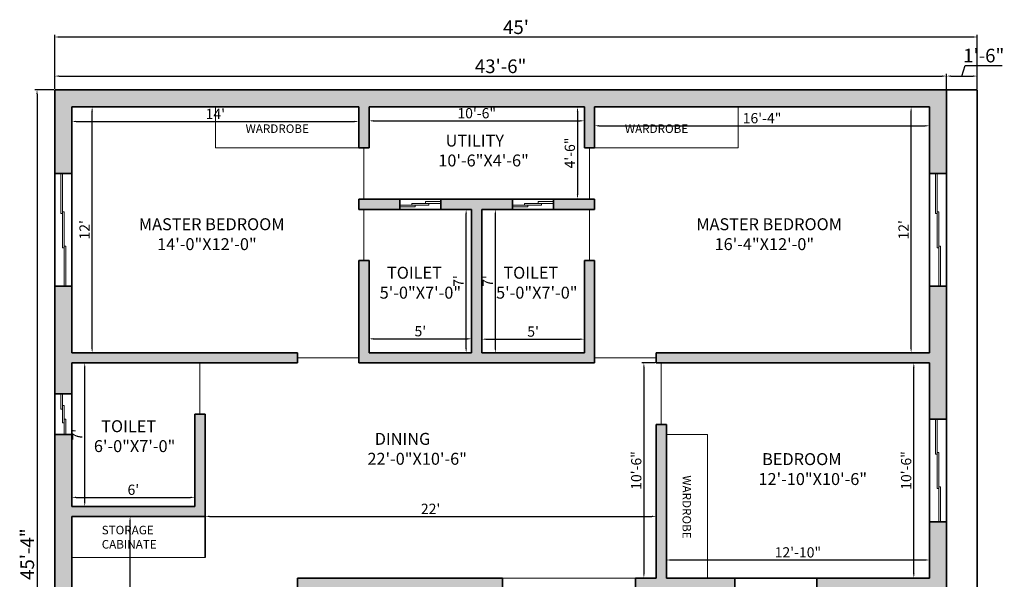
# Model space of a CAD drawing. Units: inches. Extents: x 3491 to 6898, y 1360 to 2019.
# Tile 7 of 9: x 5693 to 6269, y 1686 to 2013. Entities that reach past the tile are written whole.
import ezdxf

# ---------------------------------------------------------------- set-up
doc = ezdxf.new("R2010")
doc.units = ezdxf.units.IN
for name, color, linetype, lineweight in [('A-ANNO-DIMS', 2, 'Continuous', 18), ('A-ANNO-TEXT', 7, 'Continuous', 18), ('A-AREA-IDEN', 7, 'Continuous', 18), ('A-DOOR', 4, 'Continuous', 18), ('A-FLOR-CASE', 8, 'Continuous', 18), ('A-GLAZ', 5, 'Continuous', 18), ('A-WALL', 7, 'Continuous', 35), ('A-WALL-PATT', 8, 'Continuous', 13)]:
    doc.layers.add(name, color=color, linetype=linetype, lineweight=lineweight)
doc.layers.add('A-WALL-OPEN', color=251, linetype='Continuous', lineweight=13, true_color=0x636466)
doc.styles.get("Standard").update_dxf_attribs({"font": 'arial.ttf'})
doc.dimstyles.new('ISO-25', dxfattribs={"dimtxt": 8, "dimasz": 2.5, "dimexe": 1.25, "dimexo": 0.625, "dimtad": 1, "dimdec": 1, "dimlunit": 3, "dimtxsty": 'Standard', "dimcen": 2.5, "dimclrt": 1, "dimadec": 0, "dimazin": 0, "dimtfac": 1, "dimtdec": 1, "dimtmove": 0, "dimatfit": 3, "dimfxl": 1, "dimarcsym": 0})

# ---------------------------------------------------------------- blocks, each defined once
blk = doc.blocks.new('*D51')
at = {"layer": 'A-ANNO-DIMS', "color": 0, "lineweight": -2, "transparency": 16777216}
for p, q in [((5713.61, 1972.99), (5713.61, 1981.69)), ((5716.11, 1980.44), (6233.11, 1980.44)), ((6235.61, 1972.99), (6235.61, 1981.69))]:
    blk.add_line(p, q, dxfattribs=at)
at = {"layer": 'A-ANNO-DIMS', "color": 0, "transparency": 16777216}
for points in [[(5716.11, 1980.85), (5716.11, 1980.02), (5713.61, 1980.44)], [(6233.11, 1980.85), (6233.11, 1980.02), (6235.61, 1980.44)]]:
    blk.add_solid(points, dxfattribs=at)
at = {"layer": 'Defpoints', "color": 0, "transparency": 16777216}
for p in [(6235.61, 1980.44), (5713.61, 1972.37), (6235.61, 1972.37)]:
    blk.add_point(p, dxfattribs=at)
at = {"layer": 'A-ANNO-DIMS', "color": 0, "transparency": 16777216, "insert": (5974.61, 1985.15), "char_height": 8, "attachment_point": 5}
blk.add_mtext('43\'-6"', dxfattribs=at)
blk = doc.blocks.new('*D52')
at = {"layer": 'A-ANNO-DIMS', "color": 0, "lineweight": -2, "transparency": 16777216}
for p, q in [((6244.61, 1980.44), (6246.49, 1986.71)), ((6246.49, 1986.71), (6268.26, 1986.71)), ((6235.61, 1972.99), (6235.61, 1981.69)), ((6238.11, 1980.44), (6251.11, 1980.44)), ((6253.61, 1972.99), (6253.61, 1981.69))]:
    blk.add_line(p, q, dxfattribs=at)
at = {"layer": 'A-ANNO-DIMS', "color": 0, "transparency": 16777216}
for points in [[(6238.11, 1980.85), (6238.11, 1980.02), (6235.61, 1980.44)], [(6251.11, 1980.85), (6251.11, 1980.02), (6253.61, 1980.44)]]:
    blk.add_solid(points, dxfattribs=at)
at = {"layer": 'Defpoints', "color": 0, "transparency": 16777216}
for p in [(6253.61, 1980.44), (6235.61, 1972.37), (6253.61, 1972.37)]:
    blk.add_point(p, dxfattribs=at)
at = {"layer": 'A-ANNO-DIMS', "color": 0, "transparency": 16777216, "insert": (6257.38, 1991.42), "char_height": 8, "attachment_point": 5}
blk.add_mtext('1\'-6"', dxfattribs=at)
blk = doc.blocks.new('*D32')
at = {"layer": 'A-ANNO-DIMS', "color": 0, "lineweight": -2, "transparency": 16777216}
for p, q in [((5713.61, 1972.99), (5713.61, 2004.59)), ((5716.11, 2003.34), (6251.11, 2003.34)), ((6253.61, 1972.99), (6253.61, 2004.59))]:
    blk.add_line(p, q, dxfattribs=at)
at = {"layer": 'A-ANNO-DIMS', "color": 0, "transparency": 16777216}
for points in [[(5716.11, 2003.76), (5716.11, 2002.92), (5713.61, 2003.34)], [(6251.11, 2003.76), (6251.11, 2002.92), (6253.61, 2003.34)]]:
    blk.add_solid(points, dxfattribs=at)
at = {"layer": 'Defpoints', "color": 0, "transparency": 16777216}
for p in [(6253.61, 2003.34), (5713.61, 1972.37), (6253.61, 1972.37)]:
    blk.add_point(p, dxfattribs=at)
at = {"layer": 'A-ANNO-DIMS', "color": 0, "transparency": 16777216, "insert": (5983.61, 2008.03), "char_height": 8, "attachment_point": 5}
blk.add_mtext("45'", dxfattribs=at)
blk = doc.blocks.new('*D53')
at = {"layer": 'A-ANNO-DIMS', "color": 0, "lineweight": -2, "transparency": 16777216}
for p, q in [((5712.99, 1972.37), (5701.98, 1972.37)), ((5703.23, 1969.87), (5703.23, 1430.87)), ((5712.99, 1428.37), (5701.98, 1428.37))]:
    blk.add_line(p, q, dxfattribs=at)
at = {"layer": 'A-ANNO-DIMS', "color": 0, "transparency": 16777216}
for points in [[(5702.81, 1969.87), (5703.65, 1969.87), (5703.23, 1972.37)], [(5702.81, 1430.87), (5703.65, 1430.87), (5703.23, 1428.37)]]:
    blk.add_solid(points, dxfattribs=at)
at = {"layer": 'Defpoints', "color": 0, "transparency": 16777216}
for p in [(5713.61, 1972.37), (5703.23, 1428.37), (5713.61, 1428.37)]:
    blk.add_point(p, dxfattribs=at)
at = {"layer": 'A-ANNO-DIMS', "color": 0, "transparency": 16777216, "insert": (5698.54, 1700.37), "char_height": 8, "attachment_point": 5, "rotation": 90}
blk.add_mtext('45\'-4"', dxfattribs=at)
blk = doc.blocks.new('*D54')
at = {"layer": 'A-ANNO-DIMS', "color": 0, "lineweight": -2, "transparency": 16777216}
for p, q in [((5723.61, 1728.99), (5723.61, 1734.88)), ((5795.61, 1728.99), (5795.61, 1734.88)), ((5726.11, 1733.63), (5793.11, 1733.63))]:
    blk.add_line(p, q, dxfattribs=at)
at = {"layer": 'A-ANNO-DIMS', "color": 0, "transparency": 16777216}
for points in [[(5726.11, 1734.05), (5726.11, 1733.21), (5723.61, 1733.63)], [(5793.11, 1734.05), (5793.11, 1733.21), (5795.61, 1733.63)]]:
    blk.add_solid(points, dxfattribs=at)
at = {"layer": 'Defpoints', "color": 0, "transparency": 16777216}
for p in [(5795.61, 1733.63), (5723.61, 1728.37), (5795.61, 1728.37)]:
    blk.add_point(p, dxfattribs=at)
at = {"layer": 'A-ANNO-DIMS', "color": 0, "transparency": 16777216, "insert": (5759.61, 1737.32), "char_height": 6, "attachment_point": 5}
blk.add_mtext("6'", dxfattribs=at)
blk = doc.blocks.new('*D55')
at = {"layer": 'A-ANNO-DIMS', "color": 0, "lineweight": -2, "transparency": 16777216}
for p, q in [((5724.24, 1812.37), (5732.4, 1812.37)), ((5731.15, 1730.87), (5731.15, 1809.87)), ((5724.24, 1728.37), (5732.4, 1728.37))]:
    blk.add_line(p, q, dxfattribs=at)
at = {"layer": 'A-ANNO-DIMS', "color": 0, "transparency": 16777216}
for points in [[(5730.73, 1809.87), (5731.57, 1809.87), (5731.15, 1812.37)], [(5730.73, 1730.87), (5731.57, 1730.87), (5731.15, 1728.37)]]:
    blk.add_solid(points, dxfattribs=at)
at = {"layer": 'Defpoints', "color": 0, "transparency": 16777216}
for p in [(5723.61, 1812.37), (5731.15, 1812.37), (5723.61, 1728.37)]:
    blk.add_point(p, dxfattribs=at)
at = {"layer": 'A-ANNO-DIMS', "color": 0, "transparency": 16777216, "insert": (5727.53, 1770.37), "char_height": 6, "attachment_point": 5, "rotation": 90}
blk.add_mtext("7'", dxfattribs=at)
blk = doc.blocks.new('*D56')
at = {"layer": 'A-ANNO-DIMS', "color": 0, "lineweight": -2, "transparency": 16777216}
for p, q in [((5724.24, 1962.37), (5736.74, 1962.37)), ((5735.49, 1820.87), (5735.49, 1959.87)), ((5724.24, 1818.37), (5736.74, 1818.37))]:
    blk.add_line(p, q, dxfattribs=at)
at = {"layer": 'A-ANNO-DIMS', "color": 0, "transparency": 16777216}
for points in [[(5735.07, 1959.87), (5735.9, 1959.87), (5735.49, 1962.37)], [(5735.07, 1820.87), (5735.9, 1820.87), (5735.49, 1818.37)]]:
    blk.add_solid(points, dxfattribs=at)
at = {"layer": 'Defpoints', "color": 0, "transparency": 16777216}
for p in [(5723.61, 1962.37), (5735.49, 1962.37), (5723.61, 1818.37)]:
    blk.add_point(p, dxfattribs=at)
at = {"layer": 'A-ANNO-DIMS', "color": 0, "transparency": 16777216, "insert": (5731.85, 1890.37), "char_height": 6, "attachment_point": 5, "rotation": 90}
blk.add_mtext("12'", dxfattribs=at)
blk = doc.blocks.new('*D57')
at = {"layer": 'A-ANNO-DIMS', "color": 0, "lineweight": -2, "transparency": 16777216}
for p, q in [((5723.61, 1961.74), (5723.61, 1952.59)), ((5891.61, 1961.74), (5891.61, 1952.59)), ((5726.11, 1953.84), (5889.11, 1953.84))]:
    blk.add_line(p, q, dxfattribs=at)
at = {"layer": 'A-ANNO-DIMS', "color": 0, "transparency": 16777216}
for points in [[(5726.11, 1954.26), (5726.11, 1953.42), (5723.61, 1953.84)], [(5889.11, 1954.26), (5889.11, 1953.42), (5891.61, 1953.84)]]:
    blk.add_solid(points, dxfattribs=at)
at = {"layer": 'Defpoints', "color": 0, "transparency": 16777216}
for p in [(5723.61, 1962.37), (5891.61, 1962.37), (5891.61, 1953.84)]:
    blk.add_point(p, dxfattribs=at)
at = {"layer": 'A-ANNO-DIMS', "color": 0, "transparency": 16777216, "insert": (5807.61, 1957.48), "char_height": 6, "attachment_point": 5}
blk.add_mtext("14'", dxfattribs=at)
blk = doc.blocks.new('*D58')
at = {"layer": 'A-ANNO-DIMS', "color": 0, "lineweight": -2, "transparency": 16777216}
for p, q in [((5897.61, 1961.74), (5897.61, 1952.97)), ((6023.61, 1961.74), (6023.61, 1952.97)), ((5900.11, 1954.22), (6021.11, 1954.22))]:
    blk.add_line(p, q, dxfattribs=at)
at = {"layer": 'A-ANNO-DIMS', "color": 0, "transparency": 16777216}
for points in [[(5900.11, 1954.64), (5900.11, 1953.81), (5897.61, 1954.22)], [(6021.11, 1954.64), (6021.11, 1953.81), (6023.61, 1954.22)]]:
    blk.add_solid(points, dxfattribs=at)
at = {"layer": 'Defpoints', "color": 0, "transparency": 16777216}
for p in [(5897.61, 1962.37), (6023.61, 1962.37), (6023.61, 1954.22)]:
    blk.add_point(p, dxfattribs=at)
at = {"layer": 'A-ANNO-DIMS', "color": 0, "transparency": 16777216, "insert": (5960.61, 1957.91), "char_height": 6, "attachment_point": 5}
blk.add_mtext('10\'-6"', dxfattribs=at)
blk = doc.blocks.new('*D59')
at = {"layer": 'A-ANNO-DIMS', "color": 0, "lineweight": -2, "transparency": 16777216}
for p, q in [((6029.61, 1961.74), (6029.61, 1950.07)), ((6225.61, 1961.74), (6225.61, 1950.07)), ((6032.11, 1951.32), (6223.11, 1951.32))]:
    blk.add_line(p, q, dxfattribs=at)
at = {"layer": 'A-ANNO-DIMS', "color": 0, "transparency": 16777216}
for points in [[(6032.11, 1951.73), (6032.11, 1950.9), (6029.61, 1951.32)], [(6223.11, 1951.73), (6223.11, 1950.9), (6225.61, 1951.32)]]:
    blk.add_solid(points, dxfattribs=at)
at = {"layer": 'Defpoints', "color": 0, "transparency": 16777216}
for p in [(6029.61, 1962.37), (6225.61, 1962.37), (6225.61, 1951.32)]:
    blk.add_point(p, dxfattribs=at)
at = {"layer": 'A-ANNO-DIMS', "color": 0, "transparency": 16777216, "insert": (6127.61, 1955), "char_height": 6, "attachment_point": 5}
blk.add_mtext('16\'-4"', dxfattribs=at)
blk = doc.blocks.new('*D60')
at = {"layer": 'A-ANNO-DIMS', "color": 0, "lineweight": -2, "transparency": 16777216}
for p, q in [((6224.99, 1962.37), (6213.63, 1962.37)), ((6214.88, 1820.87), (6214.88, 1959.87)), ((6224.99, 1818.37), (6213.63, 1818.37))]:
    blk.add_line(p, q, dxfattribs=at)
at = {"layer": 'A-ANNO-DIMS', "color": 0, "transparency": 16777216}
for points in [[(6214.47, 1959.87), (6215.3, 1959.87), (6214.88, 1962.37)], [(6214.47, 1820.87), (6215.3, 1820.87), (6214.88, 1818.37)]]:
    blk.add_solid(points, dxfattribs=at)
at = {"layer": 'Defpoints', "color": 0, "transparency": 16777216}
for p in [(6214.88, 1962.37), (6225.61, 1962.37), (6225.61, 1818.37)]:
    blk.add_point(p, dxfattribs=at)
at = {"layer": 'A-ANNO-DIMS', "color": 0, "transparency": 16777216, "insert": (6211.25, 1890.37), "char_height": 6, "attachment_point": 5, "rotation": 90}
blk.add_mtext("12'", dxfattribs=at)
blk = doc.blocks.new('*D61')
at = {"layer": 'A-ANNO-DIMS', "color": 0, "lineweight": -2, "transparency": 16777216}
for p, q in [((6071.61, 1686.99), (6071.61, 1698.19)), ((6074.11, 1696.94), (6223.11, 1696.94)), ((6225.61, 1686.99), (6225.61, 1698.19))]:
    blk.add_line(p, q, dxfattribs=at)
at = {"layer": 'A-ANNO-DIMS', "color": 0, "transparency": 16777216}
for points in [[(6074.11, 1697.36), (6074.11, 1696.53), (6071.61, 1696.94)], [(6223.11, 1697.36), (6223.11, 1696.53), (6225.61, 1696.94)]]:
    blk.add_solid(points, dxfattribs=at)
at = {"layer": 'Defpoints', "color": 0, "transparency": 16777216}
for p in [(6225.61, 1696.94), (6071.61, 1686.37), (6225.61, 1686.37)]:
    blk.add_point(p, dxfattribs=at)
at = {"layer": 'A-ANNO-DIMS', "color": 0, "transparency": 16777216, "insert": (6148.61, 1700.63), "char_height": 6, "attachment_point": 5}
blk.add_mtext('12\'-10"', dxfattribs=at)
blk = doc.blocks.new('*D62')
at = {"layer": 'A-ANNO-DIMS', "color": 0, "lineweight": -2, "transparency": 16777216}
for p, q in [((6224.99, 1812.37), (6215.2, 1812.37)), ((6216.45, 1688.87), (6216.45, 1809.87)), ((6224.99, 1686.37), (6215.2, 1686.37))]:
    blk.add_line(p, q, dxfattribs=at)
at = {"layer": 'A-ANNO-DIMS', "color": 0, "transparency": 16777216}
for points in [[(6216.03, 1809.87), (6216.87, 1809.87), (6216.45, 1812.37)], [(6216.03, 1688.87), (6216.87, 1688.87), (6216.45, 1686.37)]]:
    blk.add_solid(points, dxfattribs=at)
at = {"layer": 'Defpoints', "color": 0, "transparency": 16777216}
for p in [(6216.45, 1812.37), (6225.61, 1812.37), (6225.61, 1686.37)]:
    blk.add_point(p, dxfattribs=at)
at = {"layer": 'A-ANNO-DIMS', "color": 0, "transparency": 16777216, "insert": (6212.76, 1749.37), "char_height": 6, "attachment_point": 5, "rotation": 90}
blk.add_mtext('10\'-6"', dxfattribs=at)
blk = doc.blocks.new('*D64')
at = {"layer": 'A-ANNO-DIMS', "color": 0, "lineweight": -2, "transparency": 16777216}
for p, q in [((5724.24, 1722.37), (5758.94, 1722.37)), ((5757.69, 1534.87), (5757.69, 1719.87)), ((5724.24, 1532.37), (5758.94, 1532.37))]:
    blk.add_line(p, q, dxfattribs=at)
at = {"layer": 'A-ANNO-DIMS', "color": 0, "transparency": 16777216}
for points in [[(5757.27, 1719.87), (5758.1, 1719.87), (5757.69, 1722.37)], [(5757.27, 1534.87), (5758.1, 1534.87), (5757.69, 1532.37)]]:
    blk.add_solid(points, dxfattribs=at)
at = {"layer": 'Defpoints', "color": 0, "transparency": 16777216}
for p in [(5723.61, 1722.37), (5757.69, 1722.37), (5723.61, 1532.37)]:
    blk.add_point(p, dxfattribs=at)
at = {"layer": 'A-ANNO-DIMS', "color": 0, "transparency": 16777216, "insert": (5754, 1627.37), "char_height": 6, "attachment_point": 5, "rotation": 90}
blk.add_mtext('15\'-10"', dxfattribs=at)
blk = doc.blocks.new('*D69')
at = {"layer": 'A-ANNO-DIMS', "color": 0, "lineweight": -2, "transparency": 16777216}
for p, q in [((5801.61, 1722.99), (5801.61, 1723.75)), ((6065.61, 1722.99), (6065.61, 1723.75)), ((5804.11, 1722.5), (6063.11, 1722.5))]:
    blk.add_line(p, q, dxfattribs=at)
at = {"layer": 'A-ANNO-DIMS', "color": 0, "transparency": 16777216}
for points in [[(5804.11, 1722.91), (5804.11, 1722.08), (5801.61, 1722.5)], [(6063.11, 1722.91), (6063.11, 1722.08), (6065.61, 1722.5)]]:
    blk.add_solid(points, dxfattribs=at)
at = {"layer": 'Defpoints', "color": 0, "transparency": 16777216}
for p in [(5801.61, 1722.37), (6065.61, 1722.5), (6065.61, 1722.37)]:
    blk.add_point(p, dxfattribs=at)
at = {"layer": 'A-ANNO-DIMS', "color": 0, "transparency": 16777216, "insert": (5933.61, 1726.14), "char_height": 6, "attachment_point": 5}
blk.add_mtext("22'", dxfattribs=at)
blk = doc.blocks.new('*D70')
at = {"layer": 'A-ANNO-DIMS', "color": 0, "lineweight": -2, "transparency": 16777216}
for p, q in [((5897.61, 1818.99), (5897.61, 1827.75)), ((5957.61, 1818.99), (5957.61, 1827.75)), ((5900.11, 1826.5), (5955.11, 1826.5))]:
    blk.add_line(p, q, dxfattribs=at)
at = {"layer": 'A-ANNO-DIMS', "color": 0, "transparency": 16777216}
for points in [[(5900.11, 1826.92), (5900.11, 1826.09), (5897.61, 1826.5)], [(5955.11, 1826.92), (5955.11, 1826.09), (5957.61, 1826.5)]]:
    blk.add_solid(points, dxfattribs=at)
at = {"layer": 'Defpoints', "color": 0, "transparency": 16777216}
for p in [(5957.61, 1826.5), (5897.61, 1818.37), (5957.61, 1818.37)]:
    blk.add_point(p, dxfattribs=at)
at = {"layer": 'A-ANNO-DIMS', "color": 0, "transparency": 16777216, "insert": (5927.61, 1830.18), "char_height": 6, "attachment_point": 5}
blk.add_mtext("5'", dxfattribs=at)
blk = doc.blocks.new('*D71')
at = {"layer": 'A-ANNO-DIMS', "color": 0, "lineweight": -2, "transparency": 16777216}
for p, q in [((5956.99, 1902.37), (5953.16, 1902.37)), ((5954.41, 1820.87), (5954.41, 1899.87)), ((5956.99, 1818.37), (5953.16, 1818.37))]:
    blk.add_line(p, q, dxfattribs=at)
at = {"layer": 'A-ANNO-DIMS', "color": 0, "transparency": 16777216}
for points in [[(5954, 1899.87), (5954.83, 1899.87), (5954.41, 1902.37)], [(5954, 1820.87), (5954.83, 1820.87), (5954.41, 1818.37)]]:
    blk.add_solid(points, dxfattribs=at)
at = {"layer": 'Defpoints', "color": 0, "transparency": 16777216}
for p in [(5954.41, 1902.37), (5957.61, 1902.37), (5957.61, 1818.37)]:
    blk.add_point(p, dxfattribs=at)
at = {"layer": 'A-ANNO-DIMS', "color": 0, "transparency": 16777216, "insert": (5950.79, 1860.37), "char_height": 6, "attachment_point": 5, "rotation": 90}
blk.add_mtext("7'", dxfattribs=at)
blk = doc.blocks.new('*D72')
at = {"layer": 'A-ANNO-DIMS', "color": 0, "lineweight": -2, "transparency": 16777216}
for p, q in [((5963.61, 1818.99), (5963.61, 1827.55)), ((6023.61, 1818.99), (6023.61, 1827.55)), ((5966.11, 1826.3), (6021.11, 1826.3))]:
    blk.add_line(p, q, dxfattribs=at)
at = {"layer": 'A-ANNO-DIMS', "color": 0, "transparency": 16777216}
for points in [[(5966.11, 1826.72), (5966.11, 1825.89), (5963.61, 1826.3)], [(6021.11, 1826.72), (6021.11, 1825.89), (6023.61, 1826.3)]]:
    blk.add_solid(points, dxfattribs=at)
at = {"layer": 'Defpoints', "color": 0, "transparency": 16777216}
for p in [(6023.61, 1826.3), (5963.61, 1818.37), (6023.61, 1818.37)]:
    blk.add_point(p, dxfattribs=at)
at = {"layer": 'A-ANNO-DIMS', "color": 0, "transparency": 16777216, "insert": (5993.61, 1829.98), "char_height": 6, "attachment_point": 5}
blk.add_mtext("5'", dxfattribs=at)
blk = doc.blocks.new('*D73')
at = {"layer": 'A-ANNO-DIMS', "color": 0, "lineweight": -2, "transparency": 16777216}
for p, q in [((5964.24, 1902.37), (5972.77, 1902.37)), ((5971.52, 1820.87), (5971.52, 1899.87)), ((5964.24, 1818.37), (5972.77, 1818.37))]:
    blk.add_line(p, q, dxfattribs=at)
at = {"layer": 'A-ANNO-DIMS', "color": 0, "transparency": 16777216}
for points in [[(5971.1, 1899.87), (5971.93, 1899.87), (5971.52, 1902.37)], [(5971.1, 1820.87), (5971.93, 1820.87), (5971.52, 1818.37)]]:
    blk.add_solid(points, dxfattribs=at)
at = {"layer": 'Defpoints', "color": 0, "transparency": 16777216}
for p in [(5963.61, 1902.37), (5971.52, 1902.37), (5963.61, 1818.37)]:
    blk.add_point(p, dxfattribs=at)
at = {"layer": 'A-ANNO-DIMS', "color": 0, "transparency": 16777216, "insert": (5967.89, 1860.37), "char_height": 6, "attachment_point": 5, "rotation": 90}
blk.add_mtext("7'", dxfattribs=at)
blk = doc.blocks.new('*D74')
at = {"layer": 'A-ANNO-DIMS', "color": 0, "lineweight": -2, "transparency": 16777216}
for p, q in [((6017.04, 1962.37), (6020.85, 1962.37)), ((6019.6, 1959.87), (6019.6, 1910.87)), ((6017.04, 1908.37), (6020.85, 1908.37))]:
    blk.add_line(p, q, dxfattribs=at)
at = {"layer": 'A-ANNO-DIMS', "color": 0, "transparency": 16777216}
for points in [[(6019.18, 1959.87), (6020.02, 1959.87), (6019.6, 1962.37)], [(6019.18, 1910.87), (6020.02, 1910.87), (6019.6, 1908.37)]]:
    blk.add_solid(points, dxfattribs=at)
at = {"layer": 'Defpoints', "color": 0, "transparency": 16777216}
for p in [(6016.42, 1962.37), (6016.42, 1908.37), (6019.6, 1908.37)]:
    blk.add_point(p, dxfattribs=at)
at = {"layer": 'A-ANNO-DIMS', "color": 0, "transparency": 16777216, "insert": (6015.91, 1935.37), "char_height": 6, "attachment_point": 5, "rotation": 90}
blk.add_mtext('4\'-6"', dxfattribs=at)
blk = doc.blocks.new('*D99')
at = {"layer": 'A-ANNO-DIMS', "color": 0, "lineweight": -2, "transparency": 16777216}
for p, q in [((6064.99, 1812.37), (6057.2, 1812.37)), ((6058.45, 1809.87), (6058.45, 1688.87)), ((6058.99, 1686.37), (6057.2, 1686.37))]:
    blk.add_line(p, q, dxfattribs=at)
at = {"layer": 'A-ANNO-DIMS', "color": 0, "transparency": 16777216}
for points in [[(6058.03, 1809.87), (6058.87, 1809.87), (6058.45, 1812.37)], [(6058.03, 1688.87), (6058.87, 1688.87), (6058.45, 1686.37)]]:
    blk.add_solid(points, dxfattribs=at)
at = {"layer": 'Defpoints', "color": 0, "transparency": 16777216}
for p in [(6065.61, 1812.37), (6058.45, 1686.37), (6059.61, 1686.37)]:
    blk.add_point(p, dxfattribs=at)
at = {"layer": 'A-ANNO-DIMS', "color": 0, "transparency": 16777216, "insert": (6054.76, 1749.37), "char_height": 6, "attachment_point": 5, "rotation": 90}
blk.add_mtext('10\'-6"', dxfattribs=at)
blk = doc.blocks.new('WIN-SLIDER-24IN')
for p, q in [((0, 1), (17, 1)), ((0, 0), (9, 0)), ((7, 1), (7, 2)), ((7, 2), (24, 2)), ((9, 0), (9, 1)), ((15, 2), (15, 3)), ((15, 3), (24, 3)), ((17, 1), (17, 2))]:
    blk.add_line(p, q)
blk = doc.blocks.new('WIN-SLIDER-66IN')
for p, q in [((0, 42.5), (0, 66)), ((1, 22.5), (1, 66)), ((1, 42.5), (0, 42.5)), ((2, 43.5), (1, 43.5)), ((2, 0), (2, 43.5)), ((3, 23.5), (2, 23.5)), ((3, 0), (3, 23.5)), ((2, 22.5), (1, 22.5))]:
    blk.add_line(p, q)
blk = doc.blocks.new('WIN-SLIDER-60IN')
for p, q in [((0, 39.5), (0, 60)), ((1, 19.5), (1, 60)), ((2, 40.5), (1, 40.5)), ((2, 0), (2, 40.5)), ((1, 39.5), (0, 39.5)), ((2, 19.5), (1, 19.5)), ((3, 20.5), (2, 20.5)), ((3, 0), (3, 20.5))]:
    blk.add_line(p, q)
blk = doc.blocks.new('WARDROBE-84X24')
for q in [(0, 84), (24, 0)]:
    blk.add_line((24, 84), q)

msp = doc.modelspace()

# ---------------------------------------------------------------- hatches: boundary and pattern name
at = {"layer": 'A-WALL-PATT'}
h = msp.add_hatch(color=256, dxfattribs=at)
h.dxf.hatch_style = 1
h.paths.add_polyline_path([(6037.61, 1532.37), (5981.61, 1532.37), (5981.61, 1522.37), (6037.61, 1522.37)])
h.paths.add_polyline_path([(6087.61, 1626.37), (6077.61, 1626.37), (6077.61, 1592.37), (6087.61, 1592.37)])
h.paths.add_polyline_path([(6087.61, 1556.37), (6077.61, 1556.37), (6077.61, 1532.37), (6073.61, 1532.37), (6073.61, 1522.37), (6087.61, 1522.37)])
h.paths.add_polyline_path([(5909.61, 1532.37), (5861.61, 1532.37), (5861.61, 1680.37), (5975.61, 1680.37), (5975.61, 1686.37), (5855.61, 1686.37), (5855.61, 1532.37), (5837.64, 1532.37), (5837.64, 1522.37), (5909.61, 1522.37)])
h.paths.add_polyline_path([(5789.64, 1532.37), (5723.61, 1532.37), (5723.61, 1580.4), (5713.61, 1580.4), (5713.61, 1428.37), (5855.61, 1428.37), (5855.61, 1438.37), (5723.61, 1438.37), (5723.61, 1522.37), (5789.64, 1522.37)])
h.paths.add_polyline_path([(5723.61, 1722.37), (5801.61, 1722.37), (5801.61, 1782.37), (5795.61, 1782.37), (5795.61, 1728.37), (5723.61, 1728.37), (5723.61, 1770.37), (5713.61, 1770.37), (5713.61, 1628.4), (5723.61, 1628.4)])
h.paths.add_polyline_path([(6087.61, 1680.37), (6111.61, 1680.37), (6111.61, 1686.37), (6071.61, 1686.37), (6071.61, 1776.37), (6065.61, 1776.37), (6065.61, 1686.37), (6053.61, 1686.37), (6053.61, 1680.37), (6077.61, 1680.37), (6077.61, 1668.37), (6087.61, 1668.37)])
h.paths.add_polyline_path([(6235.61, 1719.37), (6225.61, 1719.37), (6225.61, 1686.37), (6159.61, 1686.37), (6159.61, 1680.37), (6235.61, 1680.37)])
h.paths.add_polyline_path([(6235.61, 1857.37), (6225.61, 1857.37), (6225.61, 1818.37), (6065.61, 1818.37), (6065.61, 1812.37), (6225.61, 1812.37), (6225.61, 1779.37), (6235.61, 1779.37)])
h.paths.add_polyline_path([(6029.61, 1872.37), (6023.61, 1872.37), (6023.61, 1818.37), (5963.61, 1818.37), (5963.61, 1902.37), (5981.61, 1902.37), (5981.61, 1908.37), (5939.61, 1908.37), (5939.61, 1902.37), (5957.61, 1902.37), (5957.61, 1818.37), (5897.61, 1818.37), (5897.61, 1872.37), (5891.61, 1872.37), (5891.61, 1812.37), (6029.61, 1812.37)])
h.paths.add_polyline_path([(5723.61, 1857.37), (5713.61, 1857.37), (5713.61, 1794.37), (5723.61, 1794.37), (5723.61, 1812.37), (5855.61, 1812.37), (5855.61, 1818.37), (5723.61, 1818.37)])
h.paths.add_polyline_path([(5723.61, 1962.37), (5891.61, 1962.37), (5891.61, 1938.37), (5897.61, 1938.37), (5897.61, 1962.37), (6023.61, 1962.37), (6023.61, 1938.37), (6029.61, 1938.37), (6029.61, 1962.37), (6225.61, 1962.37), (6225.61, 1923.37), (6235.61, 1923.37), (6235.61, 1972.37), (5713.61, 1972.37), (5713.61, 1923.37), (5723.61, 1923.37)])
h.paths.add_polyline_path([(5915.61, 1908.37), (5891.61, 1908.37), (5891.61, 1902.37), (5915.61, 1902.37)])
h.paths.add_polyline_path([(6029.61, 1908.37), (6005.61, 1908.37), (6005.61, 1902.37), (6029.61, 1902.37)], flags=17)

# ---------------------------------------------------------------- linework, layer by layer
at = {"layer": 'A-DOOR'}
for p, q in [((5894.61, 1938.37), (5894.61, 1908.37)), ((6026.61, 1938.37), (6026.61, 1908.37)), ((5894.61, 1872.37), (5894.61, 1902.37)), ((6026.61, 1872.37), (6026.61, 1902.37)), ((5798.61, 1782.37), (5798.61, 1812.37)), ((5855.61, 1815.37), (5891.61, 1815.37)), ((6065.61, 1815.37), (6029.61, 1815.37)), ((6068.61, 1776.37), (6068.61, 1812.37))]:
    msp.add_line(p, q, dxfattribs=at)
at = {"layer": 'A-FLOR-CASE'}
for p, q in [((5807.61, 1962.37), (5807.61, 1938.37)), ((6113.61, 1962.37), (6113.61, 1938.37)), ((5897.61, 1938.37), (5807.61, 1938.37)), ((6113.61, 1938.37), (6023.61, 1938.37)), ((5801.61, 1698.37), (5723.61, 1698.37))]:
    msp.add_line(p, q, dxfattribs=at)
at = {"layer": 'A-WALL'}
for p, q in [((6253.61, 1972.37), (5713.61, 1972.37)), ((5713.61, 1972.37), (5713.61, 1428.37)), ((6235.61, 1972.37), (6235.61, 1621.37)), ((6253.61, 1428.37), (6253.61, 1972.37)), ((5891.61, 1962.37), (5723.61, 1962.37)), ((5723.61, 1962.37), (5723.61, 1818.37)), ((5891.61, 1962.37), (5891.61, 1938.37)), ((6023.61, 1962.37), (5897.61, 1962.37)), ((5897.61, 1962.37), (5897.61, 1938.37)), ((6023.61, 1962.37), (6023.61, 1938.37)), ((6225.61, 1962.37), (6029.61, 1962.37)), ((6029.61, 1962.37), (6029.61, 1938.37)), ((6225.61, 1962.37), (6225.61, 1818.37)), ((5897.61, 1938.37), (5891.61, 1938.37)), ((6029.61, 1938.37), (6023.61, 1938.37)), ((5723.61, 1923.37), (5713.61, 1923.37)), ((6235.61, 1923.37), (6225.61, 1923.37)), ((5891.61, 1908.37), (5891.61, 1902.37)), ((6029.61, 1908.37), (5891.61, 1908.37)), ((5915.61, 1908.37), (5915.61, 1902.37)), ((5939.61, 1908.37), (5939.61, 1902.37)), ((5981.61, 1908.37), (5981.61, 1902.37)), ((6005.61, 1908.37), (6005.61, 1902.37)), ((6029.61, 1908.37), (6029.61, 1902.37)), ((5957.61, 1902.37), (5891.61, 1902.37)), ((5957.61, 1902.37), (5957.61, 1818.37)), ((5963.61, 1902.37), (5963.61, 1818.37)), ((6029.61, 1902.37), (5963.61, 1902.37)), ((5891.61, 1872.37), (5891.61, 1812.37)), ((5897.61, 1872.37), (5891.61, 1872.37)), ((5897.61, 1872.37), (5897.61, 1818.37)), ((6023.61, 1872.37), (6023.61, 1818.37)), ((6029.61, 1872.37), (6023.61, 1872.37)), ((6029.61, 1872.37), (6029.61, 1812.37)), ((5723.61, 1857.37), (5713.61, 1857.37)), ((6235.61, 1857.37), (6225.61, 1857.37)), ((5855.61, 1818.37), (5723.61, 1818.37)), ((5855.61, 1818.37), (5855.61, 1812.37)), ((5957.61, 1818.37), (5897.61, 1818.37)), ((6023.61, 1818.37), (5963.61, 1818.37)), ((6225.61, 1818.37), (6065.61, 1818.37)), ((6065.61, 1818.37), (6065.61, 1812.37)), ((5855.61, 1812.37), (5723.61, 1812.37)), ((5723.61, 1812.37), (5723.61, 1728.37)), ((6029.61, 1812.37), (5891.61, 1812.37)), ((6225.61, 1812.37), (6065.61, 1812.37)), ((6225.61, 1812.37), (6225.61, 1686.37)), ((5723.61, 1794.37), (5713.61, 1794.37)), ((5801.61, 1782.37), (5795.61, 1782.37)), ((5795.61, 1782.37), (5795.61, 1728.37)), ((5801.61, 1782.37), (5801.61, 1698.37)), ((6071.61, 1776.37), (6065.61, 1776.37)), ((6065.61, 1776.37), (6065.61, 1686.37)), ((6071.61, 1776.37), (6071.61, 1686.37)), ((6235.61, 1779.37), (6225.61, 1779.37)), ((5723.61, 1770.37), (5713.61, 1770.37)), ((5795.61, 1728.37), (5723.61, 1728.37)), ((5801.61, 1722.37), (5723.61, 1722.37)), ((5723.61, 1722.37), (5723.61, 1532.37)), ((6235.61, 1719.37), (6225.61, 1719.37)), ((5975.61, 1686.37), (5855.61, 1686.37)), ((5855.61, 1686.37), (5855.61, 1532.37)), ((5975.61, 1686.37), (5975.61, 1680.37)), ((6065.61, 1686.37), (6053.61, 1686.37)), ((6053.61, 1686.37), (6053.61, 1680.37)), ((6225.61, 1686.37), (6071.61, 1686.37)), ((6111.61, 1686.37), (6111.61, 1680.37)), ((6159.61, 1686.37), (6159.61, 1680.37))]:
    msp.add_line(p, q, dxfattribs=at)
at = {"layer": 'A-WALL-OPEN'}
msp.add_line((6053.61, 1686.37), (5975.61, 1686.37), dxfattribs=at)

# ---------------------------------------------------------------- block references
at = {"layer": 'A-FLOR-CASE'}
msp.add_blockref('WARDROBE-84X24', (6071.61, 1686.37), dxfattribs=at)
at = {"layer": 'A-GLAZ'}
for name, p in [('WIN-SLIDER-66IN', (5717.11, 1857.37)), ('WIN-SLIDER-66IN', (6229.11, 1857.37)), ('WIN-SLIDER-24IN', (5915.61, 1903.87)), ('WIN-SLIDER-24IN', (5981.61, 1903.87)), ('WIN-SLIDER-60IN', (6229.11, 1719.37))]:
    msp.add_blockref(name, p, dxfattribs=at)
at = {"layer": 'A-GLAZ', "rotation": 270}
msp.add_blockref('WIN-SLIDER-24IN', (5717.11, 1794.37), dxfattribs=at)

# ---------------------------------------------------------------- texts
at = {"layer": 'A-ANNO-TEXT', "char_height": 5, "attachment_point": 1}
for s, insert in [('WARDROBE', (5825.32, 1952.13)), ('WARDROBE', (6047.32, 1952.13)), ('STORAGE\\PCABINATE', (5741.1, 1716.98))]:
    msp.add_mtext_dynamic_manual_height_columns(s, width=86.9528, gutter_width=12.5, heights=[0], dxfattribs=dict(at, insert=insert))
at = {"layer": 'A-ANNO-TEXT', "insert": (6086.06, 1746.53), "char_height": 5, "attachment_point": 1, "rotation": 270}
msp.add_mtext_dynamic_manual_height_columns('WARDROBE', width=86.9528, gutter_width=12.5, heights=[0], dxfattribs=at)
at = {"layer": 'A-AREA-IDEN', "char_height": 7, "attachment_point": 1}
for s, heights, insert in [('  UTILITY\\P10\'-6"X4\'-6"', [0], (5938.12, 1946.16)), ('MASTER BEDROOM\\P     14\'-0"X12\'-0"', [0], (5762.85, 1897.15)), ('MASTER BEDROOM\\P     16\'-4"X12\'-0"', [0], (6089.14, 1897.15)), ('  TOILET\\P5\'-0"X7\'-0"', [0], (5903.8, 1868.72)), ('  TOILET\\P5\'-0"X7\'-0"', [0], (5971.94, 1868.72)), ('  TOILET\\P6\'-0"X7\'-0"', [0], (5736.52, 1778.82)), ('  DINING\\P22\'-0"X10\'-6"', [18.93], (5896.62, 1771.4)), (' BEDROOM\\P12\'-10"X10\'-6"', [0], (6125.53, 1759.53))]:
    msp.add_mtext_dynamic_manual_height_columns(s, width=121.6144, gutter_width=12.5, heights=heights, dxfattribs=dict(at, insert=insert))

# ---------------------------------------------------------------- dimensions: what is measured, and where the dimension line sits
at = {"layer": 'A-ANNO-DIMS'}
for base, p1, p2, override, picture, middle in [((6253.61, 2003.34), (5713.61, 1972.37), (6253.61, 1972.37), {"dimclrd": 0, "dimclre": 0, "dimclrt": 0}, '*D32', (5983.61, 2008.03)), ((6253.61, 1980.44), (6235.61, 1972.37), (6253.61, 1972.37), {"dimclrd": 0, "dimclre": 0, "dimclrt": 0, "dimtmove": 1}, '*D52', (6247.12, 1991.42)), ((6235.61, 1980.44), (5713.61, 1972.37), (6235.61, 1972.37), {"dimclrd": 0, "dimclre": 0, "dimclrt": 0}, '*D51', (5974.61, 1985.15)), ((5891.61, 1953.84), (5723.61, 1962.37), (5891.61, 1962.37), {"dimtxt": 6, "dimclrd": 0, "dimclre": 0, "dimclrt": 0}, '*D57', (5807.61, 1957.48)), ((6023.61, 1954.22), (5897.61, 1962.37), (6023.61, 1962.37), {"dimtxt": 6, "dimclrd": 0, "dimclre": 0, "dimclrt": 0}, '*D58', (5960.61, 1957.91)), ((6225.61, 1951.32), (6029.61, 1962.37), (6225.61, 1962.37), {"dimtxt": 6, "dimclrd": 0, "dimclre": 0, "dimclrt": 0}, '*D59', (6127.61, 1955)), ((5957.61, 1826.5), (5897.61, 1818.37), (5957.61, 1818.37), {"dimtxt": 6, "dimclrd": 0, "dimclre": 0, "dimclrt": 0}, '*D70', (5927.61, 1830.18)), ((6023.61, 1826.3), (5963.61, 1818.37), (6023.61, 1818.37), {"dimtxt": 6, "dimclrd": 0, "dimclre": 0, "dimclrt": 0}, '*D72', (5993.61, 1829.98)), ((5795.61, 1733.63), (5723.61, 1728.37), (5795.61, 1728.37), {"dimtxt": 6, "dimclrd": 0, "dimclre": 0, "dimclrt": 0}, '*D54', (5759.61, 1737.32)), ((6065.61, 1722.5), (5801.61, 1722.37), (6065.61, 1722.37), {"dimtxt": 6, "dimclrd": 0, "dimclre": 0, "dimclrt": 0}, '*D69', (5933.61, 1726.14)), ((6225.61, 1696.94), (6071.61, 1686.37), (6225.61, 1686.37), {"dimtxt": 6, "dimclrd": 0, "dimclre": 0, "dimclrt": 0}, '*D61', (6148.61, 1700.63))]:
    dim = msp.add_linear_dim(base=base, p1=p1, p2=p2, dimstyle='ISO-25', override=override, dxfattribs=at)
    dim.commit()
    dim.dimension.update_dxf_attribs({"geometry": picture, "text_midpoint": middle})
for base, p1, p2, angle, override, picture, middle in [((5703.23, 1428.37), (5713.61, 1972.37), (5713.61, 1428.37), 90, {"dimclrd": 0, "dimclre": 0, "dimclrt": 0}, '*D53', (5698.54, 1700.37)), ((5735.49, 1962.37), (5723.61, 1818.37), (5723.61, 1962.37), 270, {"dimtxt": 6, "dimclrd": 0, "dimclre": 0, "dimclrt": 0}, '*D56', (5731.85, 1890.37)), ((6019.6, 1908.37), (6016.42, 1962.37), (6016.42, 1908.37), 90, {"dimtxt": 6, "dimclrd": 0, "dimclre": 0, "dimclrt": 0}, '*D74', (6015.91, 1935.37)), ((6214.88, 1962.37), (6225.61, 1818.37), (6225.61, 1962.37), 270, {"dimtxt": 6, "dimclrd": 0, "dimclre": 0, "dimclrt": 0}, '*D60', (6211.25, 1890.37)), ((5954.41, 1902.37), (5957.61, 1818.37), (5957.61, 1902.37), 270, {"dimtxt": 6, "dimclrd": 0, "dimclre": 0, "dimclrt": 0}, '*D71', (5950.79, 1860.37)), ((5971.52, 1902.37), (5963.61, 1818.37), (5963.61, 1902.37), 270, {"dimtxt": 6, "dimclrd": 0, "dimclre": 0, "dimclrt": 0}, '*D73', (5967.89, 1860.37)), ((5731.15, 1812.37), (5723.61, 1728.37), (5723.61, 1812.37), 270, {"dimtxt": 6, "dimclrd": 0, "dimclre": 0, "dimclrt": 0}, '*D55', (5727.53, 1770.37)), ((6058.45, 1686.37), (6065.61, 1812.37), (6059.61, 1686.37), 90, {"dimtxt": 6, "dimclrd": 0, "dimclre": 0, "dimclrt": 0}, '*D99', (6054.76, 1749.37)), ((6216.45, 1812.37), (6225.61, 1686.37), (6225.61, 1812.37), 270, {"dimtxt": 6, "dimclrd": 0, "dimclre": 0, "dimclrt": 0}, '*D62', (6212.76, 1749.37)), ((5757.69, 1722.37), (5723.61, 1532.37), (5723.61, 1722.37), 270, {"dimtxt": 6, "dimclrd": 0, "dimclre": 0, "dimclrt": 0}, '*D64', (5754, 1627.37))]:
    dim = msp.add_linear_dim(base=base, p1=p1, p2=p2, angle=angle, dimstyle='ISO-25', override=override, dxfattribs=at)
    dim.commit()
    dim.dimension.update_dxf_attribs({"geometry": picture, "text_midpoint": middle})

doc.saveas('drawing.dxf')
